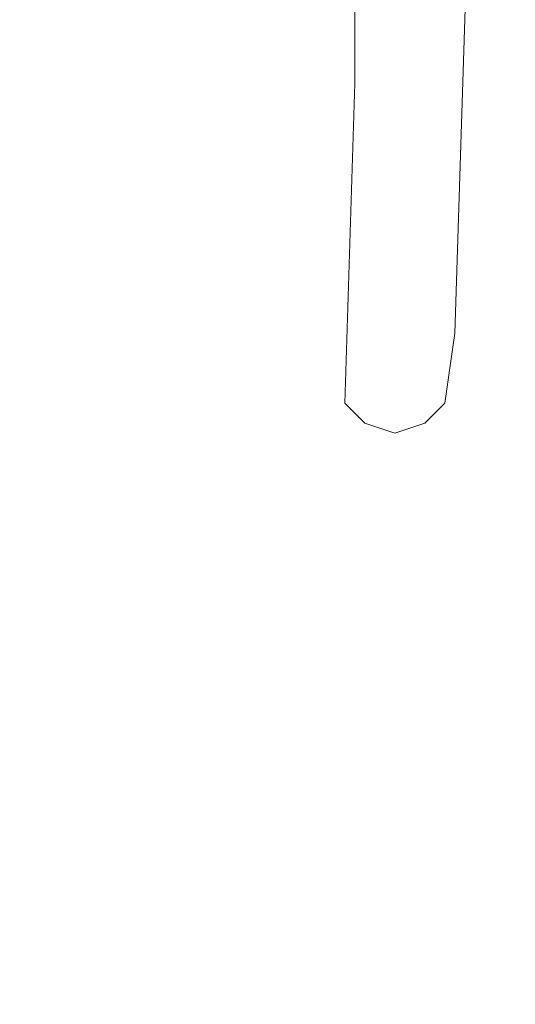
# Model space of a CAD drawing. Units: inches. Extents: x 375 to 1122, y 27 to 1069.
# Tile 126 of 155: x 717.617 to 720.668, y 900.211 to 906.27. Entities that reach past the tile are written whole.
import ezdxf

# ---------------------------------------------------------------- set-up
doc = ezdxf.new("R2010")
doc.units = ezdxf.units.IN
doc.layers.add('A-ANNO-DIMS', color=2, linetype='Continuous', lineweight=18)
doc.layers.add('Furniture', color=30, linetype='Continuous', lineweight=18)
doc.styles.get("Standard").update_dxf_attribs({"font": 'arial.ttf'})
doc.dimstyles.new('ISO-25', dxfattribs={"dimtxt": 12, "dimasz": 2.5, "dimexe": 1.5, "dimexo": 1.5, "dimtad": 1, "dimdec": 1, "dimlunit": 3, "dimtxsty": 'Standard', "dimblk": 'ARCHTICK', "dimcen": 2.5, "dimadec": 0, "dimazin": 0, "dimtfac": 1, "dimtdec": 1, "dimtmove": 0, "dimatfit": 3, "dimfxl": 1.5, "dimfxlon": 1, "dimarcsym": 0})

# ---------------------------------------------------------------- blocks, each defined once
blk = doc.blocks.new('A$C403C54AD')
for points, invisible_edges in [([(0.81108, 0.86831, -0.03586), (0.84956, 0.8837, -0.03586), (0.75259, 0.88678, -0.03586), (0.75259, 0.86831, -0.03586)], 5), ([(0.81108, 0.86831, -0.0374), (0.84956, 0.8837, -0.0374), (0.75259, 0.88678, -0.0374), (0.75259, 0.86831, -0.0374)], 5), ([(0.84956, 0.8837, -0.0374), (0.84956, 0.8837, -0.03586), (0.75259, 0.88678, -0.03586), (0.75259, 0.88678, -0.0374)], 5), ([(0.86033, 0.88216, -0.03586), (0.86033, 0.86677, -0.03586), (0.81108, 0.86831, -0.03586), (0.84956, 0.8837, -0.03586)], 5), ([(0.86033, 0.88216, -0.0374), (0.86033, 0.86677, -0.0374), (0.81108, 0.86831, -0.0374), (0.84956, 0.8837, -0.0374)], 5), ([(0.86033, 0.88216, -0.03586), (0.86033, 0.88216, -0.0374), (0.84956, 0.8837, -0.0374), (0.84956, 0.8837, -0.03586)], 5), ([(0.86341, 0.86985, -0.03586), (0.86341, 0.87908, -0.03586), (0.86033, 0.88216, -0.03586), (0.86033, 0.86677, -0.03586)], 5), ([(0.86341, 0.86985, -0.0374), (0.86341, 0.87908, -0.0374), (0.86033, 0.88216, -0.0374), (0.86033, 0.86677, -0.0374)], 5), ([(0.86341, 0.87908, -0.0374), (0.86341, 0.87908, -0.03586), (0.86033, 0.88216, -0.03586), (0.86033, 0.88216, -0.0374)], 5), ([(0.86495, 0.87446, -0.03586), (0.86495, 0.87446, -0.03586), (0.86341, 0.86985, -0.03586), (0.86341, 0.87908, -0.03586)], 4), ([(0.86495, 0.87446, -0.0374), (0.86495, 0.87446, -0.0374), (0.86341, 0.86985, -0.0374), (0.86341, 0.87908, -0.0374)], 4), ([(0.86495, 0.87446, -0.03586), (0.86495, 0.87446, -0.0374), (0.86341, 0.87908, -0.0374), (0.86341, 0.87908, -0.03586)], 4), ([(0.86341, 0.86985, -0.0374), (0.86341, 0.86985, -0.03586), (0.86495, 0.87446, -0.03586), (0.86495, 0.87446, -0.0374)], 1), ([(0.86033, 0.86677, -0.03586), (0.86033, 0.86677, -0.0374), (0.86341, 0.86985, -0.0374), (0.86341, 0.86985, -0.03586)], 5), ([(0.75259, 0.86831, -0.03586), (0.75259, 0.86831, -0.0374), (0.81108, 0.86831, -0.0374), (0.81108, 0.86831, -0.03586)], 5), ([(0.81108, 0.86831, -0.0374), (0.81108, 0.86831, -0.03586), (0.86033, 0.86677, -0.03586), (0.86033, 0.86677, -0.0374)], 5)]:
    blk.add_3dface(points, dxfattribs=dict(invisible_edges=invisible_edges))
blk = doc.blocks.new('_ArchTick')
at = {"color": 0, "linetype": 'ByBlock', "const_width": 0.15}
blk.add_lwpolyline([(-0.5, -0.5), (0.5, 0.5)], dxfattribs=at)
blk = doc.blocks.new('*D73')
at = {"layer": 'A-ANNO-DIMS', "color": 0, "lineweight": -2, "transparency": 16777216}
for p, q in [((686.7573, 932.4277), (686.7573, 929.4277)), ((770.7573, 932.4277), (770.7573, 929.4277)), ((686.7573, 930.9277), (770.7573, 930.9277)), ((770.7573, 930.9277), (987.6096, 930.9277))]:
    blk.add_line(p, q, dxfattribs=at)
at = {"layer": 'Defpoints', "color": 0, "transparency": 16777216}
for p in [(686.7573, 943.5277), (770.7573, 943.5277), (770.7573, 930.9277)]:
    blk.add_point(p, dxfattribs=at)
at = {"layer": 'A-ANNO-DIMS', "color": 0, "lineweight": -2, "transparency": 16777216, "xscale": 2.5, "yscale": 2.5, "zscale": 2.5, "rotation": 180}
blk.add_blockref('_ArchTick', (686.7573, 930.9277), dxfattribs=at)
at = {"layer": 'A-ANNO-DIMS', "color": 0, "lineweight": -2, "transparency": 16777216, "xscale": 2.5, "yscale": 2.5, "zscale": 2.5}
blk.add_blockref('_ArchTick', (770.7573, 930.9277), dxfattribs=at)
at = {"layer": 'A-ANNO-DIMS', "color": 0, "transparency": 16777216, "insert": (880.4335, 937.7573), "char_height": 12, "attachment_point": 5}
blk.add_mtext('2-PANEL SLIDER 7\'-0" TYP.', dxfattribs=at)

msp = doc.modelspace()

# ---------------------------------------------------------------- block references
at = {"layer": 'Furniture', "xscale": 39.9918517141215, "yscale": 39.9918517141215, "zscale": 39.9918517141215, "rotation": 270}
msp.add_blockref('A$C403C54AD', (684.9549, 938.3156, 0.024), dxfattribs=at)

# ---------------------------------------------------------------- dimensions: what is measured, and where the dimension line sits
at = {"layer": 'A-ANNO-DIMS'}
dim = msp.add_linear_dim(base=(770.7573, 930.9277), p1=(686.7573, 943.5277), p2=(770.7573, 943.5277), text='2-PANEL SLIDER <> TYP.', dimstyle='ISO-25', override={"dimdec": 1, "dimlfac": 1, "dimrnd": 0, "dimzin": 1, "dimdsep": 46, "dimlunit": 4, "dimfrac": 2}, dxfattribs=at)
dim.commit()
dim.dimension.update_dxf_attribs({"geometry": '*D73', "text_midpoint": (880.4335, 937.7573)})

doc.saveas('drawing.dxf')
